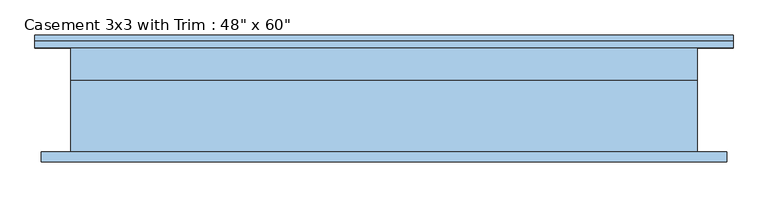
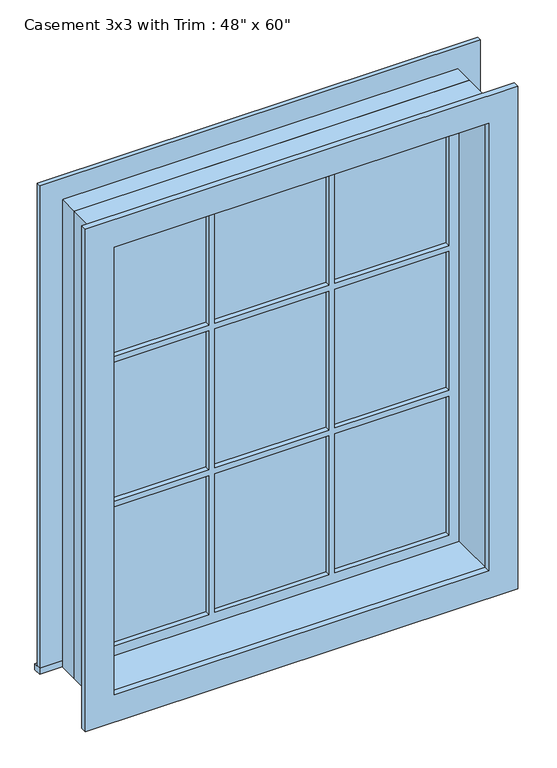
"""IFC4 building model written with IfcOpenShell, lengths in millimetres: window geometry."""

from ifc_helpers import new_model, si_unit, frame, origin, place, context, project, spatial, polyline, outline, extrude, source, transform, mapped, element, save


def window_99fc0ff6(model_context):
    return source(origin(), model_context, "Body", "SweptSolid", [
        extrude(outline(polyline([(-679.45, 127.0), (679.45, 127.0), (679.45, 101.6), (-679.45, 101.6), (-679.45, 127.0)])), frame((0.0, 0.0, 304.8), z_axis=(0.0, 0.0, 1.0), x_axis=(1.0, 0.0, 0.0)), (0.0, 0.0, 1.0), 19.05),
        extrude(outline(polyline([(1809.75, -590.55), (1809.75, 590.55), (323.85, 590.55), (323.85, 679.45), (1898.65, 679.45), (1898.65, -679.45), (323.85, -679.45), (323.85, -590.55), (1809.75, -590.55)])), frame((0.0, 101.6, 0.0), z_axis=(0.0, 1.0, 0.0), x_axis=(0.0, 0.0, 1.0)), (0.0, 0.0, 1.0), 12.7),
        extrude(outline(polyline([(194.7333333, 66.675), (546.1, 66.675), (546.1, 53.975), (194.7333333, 53.975), (194.7333333, 66.675)])), frame((0.0, 0.0, 1312.3333333), z_axis=(0.0, 0.0, 1.0), x_axis=(1.0, 0.0, 0.0)), (0.0, 0.0, 1.0), 452.9666667),
        extrude(outline(polyline([(-175.6833333, 66.675), (175.6833333, 66.675), (175.6833333, 53.975), (-175.6833333, 53.975), (-175.6833333, 66.675)])), frame((0.0, 0.0, 1312.3333333), z_axis=(0.0, 0.0, 1.0), x_axis=(1.0, 0.0, 0.0)), (0.0, 0.0, 1.0), 452.9666667),
        extrude(outline(polyline([(-546.1, 66.675), (-194.7333333, 66.675), (-194.7333333, 53.975), (-546.1, 53.975), (-546.1, 66.675)])), frame((0.0, 0.0, 1312.3333333), z_axis=(0.0, 0.0, 1.0), x_axis=(1.0, 0.0, 0.0)), (0.0, 0.0, 1.0), 452.9666667),
        extrude(outline(polyline([(-546.1, 66.675), (-194.7333333, 66.675), (-194.7333333, 53.975), (-546.1, 53.975), (-546.1, 66.675)])), frame((0.0, 0.0, 840.3166667), z_axis=(0.0, 0.0, 1.0), x_axis=(1.0, 0.0, 0.0)), (0.0, 0.0, 1.0), 452.9666667),
        extrude(outline(polyline([(-175.6833333, 66.675), (175.6833333, 66.675), (175.6833333, 53.975), (-175.6833333, 53.975), (-175.6833333, 66.675)])), frame((0.0, 0.0, 840.3166667), z_axis=(0.0, 0.0, 1.0), x_axis=(1.0, 0.0, 0.0)), (0.0, 0.0, 1.0), 452.9666667),
        extrude(outline(polyline([(194.7333333, 66.675), (546.1, 66.675), (546.1, 53.975), (194.7333333, 53.975), (194.7333333, 66.675)])), frame((0.0, 0.0, 840.3166667), z_axis=(0.0, 0.0, 1.0), x_axis=(1.0, 0.0, 0.0)), (0.0, 0.0, 1.0), 452.9666667),
        extrude(outline(polyline([(194.7333333, 66.675), (546.1, 66.675), (546.1, 53.975), (194.7333333, 53.975), (194.7333333, 66.675)])), frame((0.0, 0.0, 368.3), z_axis=(0.0, 0.0, 1.0), x_axis=(1.0, 0.0, 0.0)), (0.0, 0.0, 1.0), 452.9666667),
        extrude(outline(polyline([(-175.6833333, 66.675), (175.6833333, 66.675), (175.6833333, 53.975), (-175.6833333, 53.975), (-175.6833333, 66.675)])), frame((0.0, 0.0, 368.3), z_axis=(0.0, 0.0, 1.0), x_axis=(1.0, 0.0, 0.0)), (0.0, 0.0, 1.0), 452.9666667),
        extrude(outline(polyline([(-546.1, 66.675), (-194.7333333, 66.675), (-194.7333333, 53.975), (-546.1, 53.975), (-546.1, 66.675)])), frame((0.0, 0.0, 368.3), z_axis=(0.0, 0.0, 1.0), x_axis=(1.0, 0.0, 0.0)), (0.0, 0.0, 1.0), 452.9666667),
        extrude(outline(polyline([(1885.95, 666.75), (1885.95, -666.75), (247.65, -666.75), (247.65, 666.75), (1885.95, 666.75)]), holes=[polyline([(1797.05, 577.85), (336.55, 577.85), (336.55, -577.85), (1797.05, -577.85), (1797.05, 577.85)])]), frame((0.0, -120.65, 0.0), z_axis=(0.0, 1.0, 0.0), x_axis=(0.0, 0.0, 1.0)), (0.0, 0.0, 1.0), 19.05),
        extrude(outline(polyline([(1809.75, -590.55), (323.85, -590.55), (323.85, 590.55), (1809.75, 590.55), (1809.75, -590.55)]), holes=[polyline([(1765.3, -194.7333333), (1312.3333333, -194.7333333), (1312.3333333, -546.1), (1765.3, -546.1), (1765.3, -194.7333333)]), polyline([(1293.2833333, -194.7333333), (840.3166667, -194.7333333), (840.3166667, -546.1), (1293.2833333, -546.1), (1293.2833333, -194.7333333)]), polyline([(821.2666667, -194.7333333), (368.3, -194.7333333), (368.3, -546.1), (821.2666667, -546.1), (821.2666667, -194.7333333)]), polyline([(1765.3, 175.6833333), (1312.3333333, 175.6833333), (1312.3333333, -175.6833333), (1765.3, -175.6833333), (1765.3, 175.6833333)]), polyline([(1293.2833333, 175.6833333), (840.3166667, 175.6833333), (840.3166667, -175.6833333), (1293.2833333, -175.6833333), (1293.2833333, 175.6833333)]), polyline([(821.2666667, 175.6833333), (368.3, 175.6833333), (368.3, -175.6833333), (821.2666667, -175.6833333), (821.2666667, 175.6833333)]), polyline([(1765.3, 546.1), (1312.3333333, 546.1), (1312.3333333, 194.7333333), (1765.3, 194.7333333), (1765.3, 546.1)]), polyline([(1293.2833333, 546.1), (840.3166667, 546.1), (840.3166667, 194.7333333), (1293.2833333, 194.7333333), (1293.2833333, 546.1)]), polyline([(821.2666667, 546.1), (368.3, 546.1), (368.3, 194.7333333), (821.2666667, 194.7333333), (821.2666667, 546.1)])]), frame((0.0, 38.1, 0.0), z_axis=(0.0, 1.0, 0.0), x_axis=(0.0, 0.0, 1.0)), (0.0, 0.0, 1.0), 44.45),
        extrude(outline(polyline([(1828.8, -609.6), (304.8, -609.6), (304.8, 609.6), (1828.8, 609.6), (1828.8, -609.6)]), holes=[polyline([(1797.05, -577.85), (1797.05, 577.85), (336.55, 577.85), (336.55, -577.85), (1797.05, -577.85)])]), frame((0.0, -101.6, 0.0), z_axis=(0.0, 1.0, 0.0), x_axis=(0.0, 0.0, 1.0)), (0.0, 0.0, 1.0), 139.7),
        extrude(outline(polyline([(1828.8, 609.6), (1828.8, -609.6), (304.8, -609.6), (304.8, 609.6), (1828.8, 609.6)]), holes=[polyline([(1809.75, 590.55), (323.85, 590.55), (323.85, -590.55), (1809.75, -590.55), (1809.75, 590.55)])]), frame((0.0, 38.1, 0.0), z_axis=(0.0, 1.0, 0.0), x_axis=(0.0, 0.0, 1.0)), (0.0, 0.0, 1.0), 63.5),
    ])


if __name__ == "__main__":
    model = new_model("IFC4")
    model_context = context("Model", 3, world=origin())
    ifc_project = project(units=[si_unit("LENGTHUNIT", "METRE", prefix="MILLI")], contexts=[model_context])
    site = spatial("IfcSite", under=ifc_project)
    building = spatial("IfcBuilding", under=site)
    placement = place(None, origin())
    window_shape = window_99fc0ff6(model_context)
    element("IfcWindow", 1, ObjectType="Casement 3x3 with Trim : 48\" x 60\"", at=placement, inside=building, context=model_context, shape_type="MappedRepresentation", body=[
        mapped(window_shape, transform((0.0, 0.0, 0.0), x_axis=(1.0, 0.0, 0.0), y_axis=(0.0, 1.0, 0.0), z_axis=(0.0, 0.0, 1.0))),
    ])
    save(model, "model.ifc")

# Revit data of these elements
# Type "Casement 3x3 with Trim : 48\" x 60\""
#   Type Mark = "12"
#   Construction Type Id = "GSP4R"
#   Assembly Code = "B2020100"
#   Analytic Construction = "1/8 in Pilkington single glazing"
#   Visual Light Transmittance = 0.9
#   Solar Heat Gain Coefficient = 0.78
#   Heat Transfer Coefficient (U) = 0.6496 BTU/(h·ft²·°F)
#   Height = 5' - 0"
#   Default Sill Height = 1' - 0"
#   Trim Projection - Ext. = 0' - 0 1/2"
#   Trim Projection - Int. = 0' - 0 3/4"
#   Trim Width - Exterior = 0' - 3 1/2"
#   Trim Width - Interior = 0' - 3 1/2"
#   Width = 4' - 0"
#   Window Inset = 0' - 0 3/4"
#   Define Thermal Properties by = 1
#   Glass Pane Material = Glass
#   Sash Material = Sash
#   Trim Exterior Material = Trim
#   Trim Interior Material = Trim
#   Wall Closure = (empty or 0)
# Element 1 (IfcWindow, "Casement 3x3 with Trim : 48\" x 60\"")
#   Materials on its faces: "Sash", "Glass", "Trim"
# Materials
#   "Glass": class "Glass", colour RGB 0 128 192, transparency 0.75, Description = "Soda Lime Glass", Cost = 0
#   "Sash": class "Wood", colour RGB 224 178 126, transparency 0
#   "Trim": class "Wood", colour RGB 224 178 126, transparency 0
